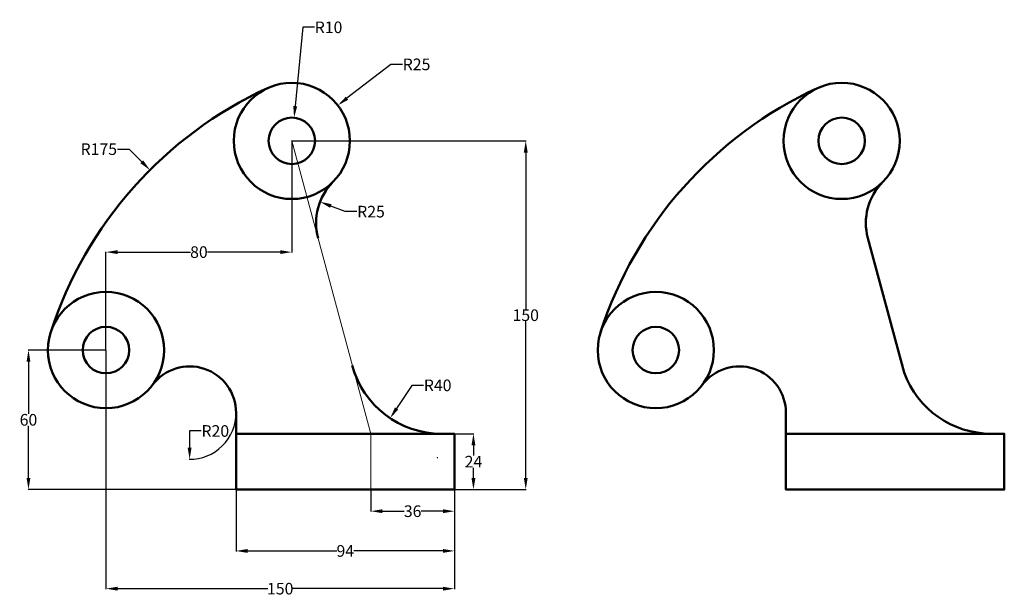
# Model space of a CAD drawing. Units: millimetres. Extents: x -71 to 353, y -37 to 211.
import ezdxf

# ---------------------------------------------------------------- set-up
doc = ezdxf.new("R2010")
doc.units = ezdxf.units.MM
doc.header["$MEASUREMENT"] = 0
for name, color, linetype, lineweight in [('M-CONS', 8, 'Continuous', 13), ('M-DIMS', 3, 'Continuous', 25), ('M-OUTL', 7, 'Continuous', 50)]:
    doc.layers.add(name, color=color, linetype=linetype, lineweight=lineweight)
doc.styles.get("Standard").update_dxf_attribs({"font": 'arial.ttf'})
doc.dimstyles.get("Standard").update_dxf_attribs({"dimtxt": 5, "dimasz": 5, "dimexe": 0.18, "dimexo": 0.0625, "dimgap": 0.09, "dimtad": 0, "dimtih": 1, "dimtoh": 1, "dimdec": 1, "dimdsep": 46, "dimtxsty": 'Standard', "dimcen": 0.09, "dimadec": 0, "dimazin": 0, "dimtfac": 1, "dimtdec": 1, "dimtofl": 0, "dimtmove": 0, "dimatfit": 3, "dimfxl": 1, "dimtolj": 1, "dimtzin": 0, "dimarcsym": 0})

# ---------------------------------------------------------------- blocks, each defined once
blk = doc.blocks.new('*D1')
at = {"layer": 'Defpoints', "color": 0, "transparency": 16777216}
for p in [(45.88, 159.31), (45.88, 9.31), (146.56, 9.31)]:
    blk.add_point(p, dxfattribs=at)
at = {"layer": 'M-DIMS', "color": 0, "lineweight": -2, "transparency": 16777216}
for p, q in [((45.95, 159.31), (146.74, 159.31)), ((146.56, 154.31), (146.56, 86.95)), ((146.56, 14.31), (146.56, 81.67)), ((45.95, 9.31), (146.74, 9.31))]:
    blk.add_line(p, q, dxfattribs=at)
at = {"layer": 'M-DIMS', "color": 0, "transparency": 16777216}
for points in [[(145.73, 154.31), (147.4, 154.31), (146.56, 159.31)], [(145.73, 14.31), (147.4, 14.31), (146.56, 9.31)]]:
    blk.add_solid(points, dxfattribs=at)
at = {"layer": 'M-DIMS', "color": 0, "transparency": 16777216, "insert": (146.56, 84.31), "char_height": 5, "attachment_point": 5}
blk.add_mtext('\\A1;150', dxfattribs=at)
blk = doc.blocks.new('*D2')
at = {"layer": 'Defpoints', "color": 0, "transparency": 16777216}
for p in [(45.88, 159.31), (45.88, 111.46), (-34.12, 69.31)]:
    blk.add_point(p, dxfattribs=at)
at = {"layer": 'M-DIMS', "color": 0, "lineweight": -2, "transparency": 16777216}
for p, q in [((45.88, 159.25), (45.88, 111.28)), ((-34.12, 69.37), (-34.12, 111.64)), ((-29.12, 111.46), (2.22, 111.46)), ((40.88, 111.46), (9.55, 111.46))]:
    blk.add_line(p, q, dxfattribs=at)
at = {"layer": 'M-DIMS', "color": 0, "transparency": 16777216}
for points in [[(-29.12, 112.29), (-29.12, 110.63), (-34.12, 111.46)], [(40.88, 112.29), (40.88, 110.63), (45.88, 111.46)]]:
    blk.add_solid(points, dxfattribs=at)
at = {"layer": 'M-DIMS', "color": 0, "transparency": 16777216, "insert": (5.88, 111.46), "char_height": 5, "attachment_point": 5}
blk.add_mtext('\\A1;80', dxfattribs=at)
blk = doc.blocks.new('*D3')
at = {"layer": 'Defpoints', "color": 0, "transparency": 16777216}
for p in [(-67.47, 69.31), (-34.12, 69.31), (21.88, 9.31)]:
    blk.add_point(p, dxfattribs=at)
at = {"layer": 'M-DIMS', "color": 0, "lineweight": -2, "transparency": 16777216}
for p, q in [((-34.18, 69.31), (-67.65, 69.31)), ((-67.47, 64.31), (-67.47, 41.95)), ((-67.47, 14.31), (-67.47, 36.67)), ((21.82, 9.31), (-67.65, 9.31))]:
    blk.add_line(p, q, dxfattribs=at)
at = {"layer": 'M-DIMS', "color": 0, "transparency": 16777216}
for points in [[(-68.3, 64.31), (-66.64, 64.31), (-67.47, 69.31)], [(-68.3, 14.31), (-66.64, 14.31), (-67.47, 9.31)]]:
    blk.add_solid(points, dxfattribs=at)
at = {"layer": 'M-DIMS', "color": 0, "transparency": 16777216, "insert": (-67.47, 39.31), "char_height": 5, "attachment_point": 5}
blk.add_mtext('\\A1;60', dxfattribs=at)
blk = doc.blocks.new('*D4')
at = {"layer": 'Defpoints', "color": 0, "transparency": 16777216}
for p in [(-34.12, 69.31), (115.88, 9.31), (115.88, -33.33)]:
    blk.add_point(p, dxfattribs=at)
at = {"layer": 'M-DIMS', "color": 0, "lineweight": -2, "transparency": 16777216}
for p, q in [((-34.12, 69.25), (-34.12, -33.51)), ((115.88, 9.25), (115.88, -33.51)), ((-29.12, -33.33), (35.51, -33.33)), ((110.88, -33.33), (46.25, -33.33))]:
    blk.add_line(p, q, dxfattribs=at)
at = {"layer": 'M-DIMS', "color": 0, "transparency": 16777216}
for points in [[(-29.12, -32.5), (-29.12, -34.17), (-34.12, -33.33)], [(110.88, -32.5), (110.88, -34.17), (115.88, -33.33)]]:
    blk.add_solid(points, dxfattribs=at)
at = {"layer": 'M-DIMS', "color": 0, "transparency": 16777216, "insert": (40.88, -33.33), "char_height": 5, "attachment_point": 5}
blk.add_mtext('\\A1;150', dxfattribs=at)
blk = doc.blocks.new('*D5')
at = {"layer": 'Defpoints', "color": 0, "transparency": 16777216}
for p in [(79.88, 9.31), (115.88, 9.31), (115.88, 0)]:
    blk.add_point(p, dxfattribs=at)
at = {"layer": 'M-DIMS', "color": 0, "lineweight": -2, "transparency": 16777216}
for p, q in [((79.88, 9.25), (79.88, -0.18)), ((115.88, 9.25), (115.88, -0.18)), ((84.88, 0), (94.22, 0)), ((110.88, 0), (101.55, 0))]:
    blk.add_line(p, q, dxfattribs=at)
at = {"layer": 'M-DIMS', "color": 0, "transparency": 16777216}
for points in [[(84.88, 0.83), (84.88, -0.84), (79.88, 0)], [(110.88, 0.83), (110.88, -0.84), (115.88, 0)]]:
    blk.add_solid(points, dxfattribs=at)
at = {"layer": 'M-DIMS', "color": 0, "transparency": 16777216, "insert": (97.88, 0), "char_height": 5, "attachment_point": 5}
blk.add_mtext('\\A1;36', dxfattribs=at)
blk = doc.blocks.new('*D6')
at = {"layer": 'Defpoints', "color": 0, "transparency": 16777216}
for p in [(21.88, 9.31), (115.88, 9.31), (115.88, -17.1)]:
    blk.add_point(p, dxfattribs=at)
at = {"layer": 'M-DIMS', "color": 0, "lineweight": -2, "transparency": 16777216}
for p, q in [((21.88, 9.25), (21.88, -17.28)), ((115.88, 9.25), (115.88, -17.28)), ((26.88, -17.1), (65.22, -17.1)), ((110.88, -17.1), (72.54, -17.1))]:
    blk.add_line(p, q, dxfattribs=at)
at = {"layer": 'M-DIMS', "color": 0, "transparency": 16777216}
for points in [[(26.88, -16.26), (26.88, -17.93), (21.88, -17.1)], [(110.88, -16.26), (110.88, -17.93), (115.88, -17.1)]]:
    blk.add_solid(points, dxfattribs=at)
at = {"layer": 'M-DIMS', "color": 0, "transparency": 16777216, "insert": (68.88, -17.1), "char_height": 5, "attachment_point": 5}
blk.add_mtext('\\A1;94', dxfattribs=at)
blk = doc.blocks.new('*D7')
at = {"layer": 'Defpoints', "color": 0, "transparency": 16777216}
for p in [(1.88, 42.31), (1.88, 22.31)]:
    blk.add_point(p, dxfattribs=at)
at = {"layer": 'M-DIMS', "color": 0, "lineweight": -2, "transparency": 16777216}
for p, q in [((6.88, 34.51), (1.88, 34.51)), ((1.88, 34.51), (1.88, 27.31))]:
    blk.add_line(p, q, dxfattribs=at)
blk.add_arc((1.88, 42.31), 20, 269.4843, 359.821, dxfattribs=at)
at = {"layer": 'M-DIMS', "color": 0, "transparency": 16777216}
blk.add_solid([(1.05, 27.31), (2.72, 27.31), (1.88, 22.31)], dxfattribs=at)
at = {"layer": 'M-DIMS', "color": 0, "transparency": 16777216, "insert": (12.94, 34.51), "char_height": 5, "attachment_point": 5}
blk.add_mtext('\\A1;R20', dxfattribs=at)
blk = doc.blocks.new('*D8')
at = {"layer": 'Defpoints', "color": 0, "transparency": 16777216}
for p in [(58.01, 133.11), (81.3, 124.02)]:
    blk.add_point(p, dxfattribs=at)
at = {"layer": 'M-DIMS', "color": 0, "lineweight": -2, "transparency": 16777216}
for p, q in [((68.86, 128.87), (62.67, 131.29)), ((73.86, 128.87), (68.86, 128.87))]:
    blk.add_line(p, q, dxfattribs=at)
at = {"layer": 'M-DIMS', "color": 0, "transparency": 16777216}
blk.add_solid([(62.97, 132.07), (62.37, 130.51), (58.01, 133.11)], dxfattribs=at)
at = {"layer": 'M-DIMS', "color": 0, "transparency": 16777216, "insert": (79.95, 128.87), "char_height": 5, "attachment_point": 5}
blk.add_mtext('\\A1;R25', dxfattribs=at)
blk = doc.blocks.new('*D9')
at = {"layer": 'Defpoints', "color": 0, "transparency": 16777216}
for p in [(110.37, 73.31), (88.19, 40.02)]:
    blk.add_point(p, dxfattribs=at)
at = {"layer": 'M-DIMS', "color": 0, "lineweight": -2, "transparency": 16777216}
for p, q in [((97.59, 54.14), (90.96, 44.18)), ((102.59, 54.14), (97.59, 54.14))]:
    blk.add_line(p, q, dxfattribs=at)
at = {"layer": 'M-DIMS', "color": 0, "transparency": 16777216}
blk.add_solid([(90.27, 44.65), (91.66, 43.72), (88.19, 40.02)], dxfattribs=at)
at = {"layer": 'M-DIMS', "color": 0, "transparency": 16777216, "insert": (108.65, 54.14), "char_height": 5, "attachment_point": 5}
blk.add_mtext('\\A1;R40', dxfattribs=at)
blk = doc.blocks.new('*D10')
at = {"layer": 'Defpoints', "color": 0, "transparency": 16777216}
for p in [(-15.18, 146.77), (108.57, 23.04)]:
    blk.add_point(p, dxfattribs=at)
at = {"layer": 'M-DIMS', "color": 0, "lineweight": -2, "transparency": 16777216}
for p, q in [((-29.18, 155.76), (-24.18, 155.76)), ((-24.18, 155.76), (-18.72, 150.31)), ((108.48, 23.04), (108.66, 23.04)), ((108.57, 22.95), (108.57, 23.13))]:
    blk.add_line(p, q, dxfattribs=at)
at = {"layer": 'M-DIMS', "color": 0, "transparency": 16777216}
blk.add_solid([(-18.13, 150.9), (-19.31, 149.72), (-15.18, 146.77)], dxfattribs=at)
at = {"layer": 'M-DIMS', "color": 0, "transparency": 16777216, "insert": (-37.2, 155.76), "char_height": 5, "attachment_point": 5}
blk.add_mtext('\\A1;R175', dxfattribs=at)
blk = doc.blocks.new('*D11')
at = {"layer": 'Defpoints', "color": 0, "transparency": 16777216}
for p in [(115.88, 33.31), (124.05, 33.31), (115.88, 9.31)]:
    blk.add_point(p, dxfattribs=at)
at = {"layer": 'M-DIMS', "color": 0, "lineweight": -2, "transparency": 16777216}
for p, q in [((115.95, 33.31), (124.23, 33.31)), ((124.05, 28.31), (124.05, 23.91)), ((124.05, 14.31), (124.05, 18.71)), ((115.95, 9.31), (124.23, 9.31))]:
    blk.add_line(p, q, dxfattribs=at)
at = {"layer": 'M-DIMS', "color": 0, "transparency": 16777216}
for points in [[(123.21, 28.31), (124.88, 28.31), (124.05, 33.31)], [(123.21, 14.31), (124.88, 14.31), (124.05, 9.31)]]:
    blk.add_solid(points, dxfattribs=at)
at = {"layer": 'M-DIMS', "color": 0, "transparency": 16777216, "insert": (124.05, 21.31), "char_height": 5, "attachment_point": 5}
blk.add_mtext('\\A1;24', dxfattribs=at)
blk = doc.blocks.new('*D12')
at = {"layer": 'Defpoints', "color": 0, "transparency": 16777216}
for p in [(46.85, 169.26), (45.88, 159.31)]:
    blk.add_point(p, dxfattribs=at)
at = {"layer": 'M-DIMS', "color": 0, "lineweight": -2, "transparency": 16777216}
for p, q in [((50.62, 208.17), (47.33, 174.24)), ((55.62, 208.17), (50.62, 208.17)), ((45.79, 159.31), (45.97, 159.31)), ((45.88, 159.22), (45.88, 159.4))]:
    blk.add_line(p, q, dxfattribs=at)
at = {"layer": 'M-DIMS', "color": 0, "transparency": 16777216}
blk.add_solid([(46.5, 174.32), (48.16, 174.16), (46.85, 169.26)], dxfattribs=at)
at = {"layer": 'M-DIMS', "color": 0, "transparency": 16777216, "insert": (61.68, 208.17), "char_height": 5, "attachment_point": 5}
blk.add_mtext('\\A1;R10', dxfattribs=at)
blk = doc.blocks.new('*D13')
at = {"layer": 'Defpoints', "color": 0, "transparency": 16777216}
for p in [(65.67, 174.59), (45.88, 159.31)]:
    blk.add_point(p, dxfattribs=at)
at = {"layer": 'M-DIMS', "color": 0, "lineweight": -2, "transparency": 16777216}
for p, q in [((88.47, 192.22), (69.62, 177.65)), ((93.47, 192.22), (88.47, 192.22)), ((45.79, 159.31), (45.97, 159.31)), ((45.88, 159.22), (45.88, 159.4))]:
    blk.add_line(p, q, dxfattribs=at)
at = {"layer": 'M-DIMS', "color": 0, "transparency": 16777216}
blk.add_solid([(69.11, 178.31), (70.13, 176.99), (65.67, 174.59)], dxfattribs=at)
at = {"layer": 'M-DIMS', "color": 0, "transparency": 16777216, "insert": (99.56, 192.22), "char_height": 5, "attachment_point": 5}
blk.add_mtext('\\A1;R25', dxfattribs=at)

msp = doc.modelspace()

# ---------------------------------------------------------------- linework, layer by layer
at = {"layer": 'M-CONS'}
for p in [(45.88, 159.31), (79.88, 9.31)]:
    msp.add_line(p, (79.88, 33.31), dxfattribs=at)
at = {"layer": 'M-OUTL'}
for p, q in [((293.82, 117.5), (309.43, 59.63)), ((21.88, 33.31), (21.88, 42.31)), ((258.54, 33.31), (258.54, 42.31)), ((115.88, 9.31), (79.88, 9.31)), ((352.54, 9.31), (316.54, 9.31))]:
    msp.add_line(p, q, dxfattribs=at)
for points in [[(21.88, 33.31), (115.88, 33.31), (115.88, 9.31), (21.88, 9.31)], [(258.54, 33.31), (352.54, 33.31), (352.54, 9.31), (258.54, 9.31)]]:
    msp.add_lwpolyline(points, close=True, dxfattribs=at)
for centre, radius in [((45.88, 159.31), 25), ((282.54, 159.31), 25), ((45.88, 159.31), 10), ((282.54, 159.31), 10), ((-34.12, 69.31), 25), ((202.54, 69.31), 25), ((-34.12, 69.31), 10), ((202.54, 69.31), 10)]:
    msp.add_circle(centre, radius, dxfattribs=at)
for centre, radius, start, end in [((108.57, 23.04), 175, 114.7016, 162.0313), ((345.22, 23.04), 175, 114.7016, 162.0313), ((81.3, 124.02), 25, 135.1011, 195.1011), ((317.95, 124.02), 25, 135.1011, 195.1011), ((1.88, 42.31), 20, 0, 143.1301), ((110.37, 73.31), 40, 195.374, 270), ((238.54, 42.31), 20, 0, 143.1301), ((347.02, 73.31), 40, 199.9925, 270)]:
    msp.add_arc(centre, radius, start, end, dxfattribs=at)

# ---------------------------------------------------------------- dimensions: what is measured, and where the dimension line sits
at = {"layer": 'M-DIMS', "transparency": 33554610}
for center, mpoint, picture, middle in [((45.88, 159.31), (46.85, 169.26), '*D12', (61.68, 208.17)), ((45.88, 159.31), (65.67, 174.59), '*D13', (99.56, 192.22)), ((108.57, 23.04), (-15.18, 146.77), '*D10', (-37.2, 155.76)), ((81.3, 124.02), (58.01, 133.11), '*D8', (79.95, 128.87)), ((110.37, 73.31), (88.19, 40.02), '*D9', (108.65, 54.14)), ((1.88, 42.31), (1.88, 22.31), '*D7', (12.94, 34.51))]:
    dim = msp.add_radius_dim(center=center, mpoint=mpoint, dimstyle='Standard', override={"dimclrd": 0, "dimclre": 0, "dimclrt": 0}, dxfattribs=at)
    dim.commit()
    dim.dimension.update_dxf_attribs({"geometry": picture, "text_midpoint": middle, "dimtype": 164})
dim = msp.add_linear_dim(base=(45.88, 111.46), p1=(-34.12, 69.31), p2=(45.88, 159.31), dimstyle='Standard', override={"dimclrd": 0, "dimclre": 0, "dimclrt": 0}, dxfattribs=at)
dim.commit()
dim.dimension.update_dxf_attribs({"geometry": '*D2', "text_midpoint": (5.88, 111.46), "dimtype": 160})
for base, p1, p2, picture, middle in [((146.56, 9.31), (45.88, 159.31), (45.88, 9.31), '*D1', (146.56, 84.31)), ((-67.47, 69.31), (21.88, 9.31), (-34.12, 69.31), '*D3', (-67.47, 39.31)), ((124.05, 33.31), (115.88, 9.31), (115.88, 33.31), '*D11', (124.05, 21.31))]:
    dim = msp.add_linear_dim(base=base, p1=p1, p2=p2, angle=90, dimstyle='Standard', override={"dimclrd": 0, "dimclre": 0, "dimclrt": 0}, dxfattribs=at)
    dim.commit()
    dim.dimension.update_dxf_attribs({"geometry": picture, "text_midpoint": middle})
for base, p1, picture, middle in [((115.88, -33.33), (-34.12, 69.31), '*D4', (40.88, -33.33)), ((115.88, -17.1), (21.88, 9.31), '*D6', (68.88, -17.1)), ((115.88, 0), (79.88, 9.31), '*D5', (97.88, 0))]:
    dim = msp.add_linear_dim(base=base, p1=p1, p2=(115.88, 9.31), dimstyle='Standard', override={"dimclrd": 0, "dimclre": 0, "dimclrt": 0}, dxfattribs=at)
    dim.commit()
    dim.dimension.update_dxf_attribs({"geometry": picture, "text_midpoint": middle})

doc.saveas('drawing.dxf')
